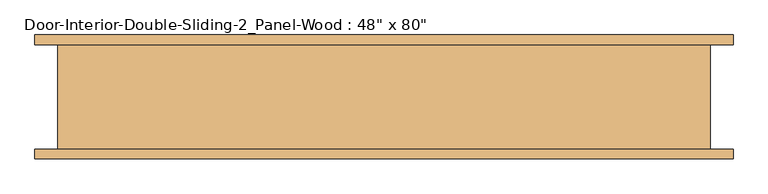
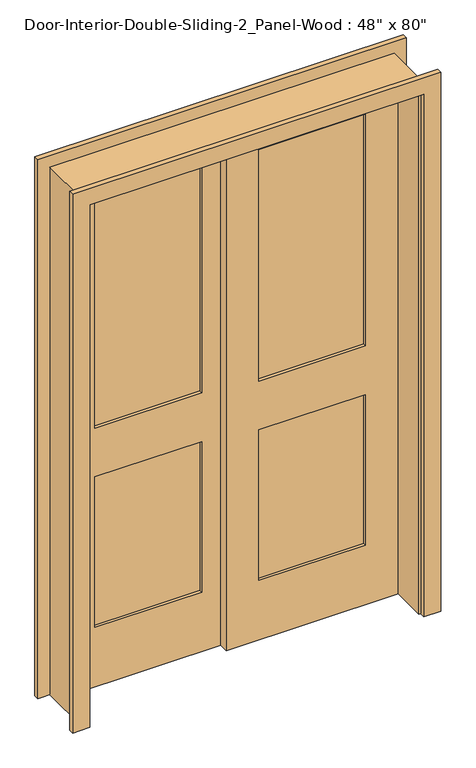
"""IFC4 building model written with IfcOpenShell, lengths in millimetres: door geometry."""

from ifc_helpers import new_model, si_unit, frame, origin, place, context, project, spatial, polyline, outline, extrude, source, transform, mapped, element, save


def door_f9cb40a9(model_context):
    return source(origin(), model_context, "Body", "SweptSolid", [
        extrude(outline(polyline([(488.95, 40.2166667), (95.25, 40.2166667), (95.25, 51.8583333), (488.95, 51.8583333), (488.95, 40.2166667)])), frame((0.0, 0.0, 1009.65), z_axis=(0.0, 0.0, 1.0), x_axis=(1.0, 0.0, 0.0)), (0.0, 0.0, 1.0), 903.2875),
        extrude(outline(polyline([(488.95, 40.2166667), (95.25, 40.2166667), (95.25, 51.8583333), (488.95, 51.8583333), (488.95, 40.2166667)])), frame((0.0, 0.0, 231.775), z_axis=(0.0, 0.0, 1.0), x_axis=(1.0, 0.0, 0.0)), (0.0, 0.0, 1.0), 587.375),
        extrude(outline(polyline([(2032.0, -25.4), (0.0, -25.4), (0.0, 609.6), (2032.0, 609.6), (2032.0, -25.4)]), holes=[polyline([(1912.9375, 95.25), (1912.9375, 488.95), (1009.65, 488.95), (1009.65, 95.25), (1912.9375, 95.25)]), polyline([(819.15, 95.25), (819.15, 488.95), (231.775, 488.95), (231.775, 95.25), (819.15, 95.25)])]), frame((0.0, 28.575, 0.0), z_axis=(0.0, 1.0, 0.0), x_axis=(0.0, 0.0, 1.0)), (0.0, 0.0, 1.0), 34.925),
        extrude(outline(polyline([(-95.25, 75.1416667), (-488.95, 75.1416667), (-488.95, 86.7833333), (-95.25, 86.7833333), (-95.25, 75.1416667)])), frame((0.0, 0.0, 1009.65), z_axis=(0.0, 0.0, 1.0), x_axis=(1.0, 0.0, 0.0)), (0.0, 0.0, 1.0), 903.2875),
        extrude(outline(polyline([(-95.25, 75.1416667), (-488.95, 75.1416667), (-488.95, 86.7833333), (-95.25, 86.7833333), (-95.25, 75.1416667)])), frame((0.0, 0.0, 231.775), z_axis=(0.0, 0.0, 1.0), x_axis=(1.0, 0.0, 0.0)), (0.0, 0.0, 1.0), 587.375),
        extrude(outline(polyline([(2032.0, -609.6), (0.0, -609.6), (0.0, 25.4), (2032.0, 25.4), (2032.0, -609.6)]), holes=[polyline([(1912.9375, -488.95), (1912.9375, -95.25), (1009.65, -95.25), (1009.65, -488.95), (1912.9375, -488.95)]), polyline([(819.15, -488.95), (819.15, -95.25), (231.775, -95.25), (231.775, -488.95), (819.15, -488.95)])]), frame((0.0, 63.5, 0.0), z_axis=(0.0, 1.0, 0.0), x_axis=(0.0, 0.0, 1.0)), (0.0, 0.0, 1.0), 34.925),
        extrude(outline(polyline([(0.0, 609.6), (0.0, 635.0), (2057.4, 635.0), (2057.4, -635.0), (0.0, -635.0), (0.0, -609.6), (2032.0, -609.6), (2032.0, 609.6), (0.0, 609.6)])), frame((0.0, -104.775, 0.0), z_axis=(0.0, 1.0, 0.0), x_axis=(0.0, 0.0, 1.0)), (0.0, 0.0, 1.0), 203.2),
        extrude(outline(polyline([(0.0, 615.95), (0.0, 679.45), (2101.85, 679.45), (2101.85, -679.45), (0.0, -679.45), (0.0, -615.95), (2038.35, -615.95), (2038.35, 615.95), (0.0, 615.95)])), frame((0.0, -123.825, 0.0), z_axis=(0.0, 1.0, 0.0), x_axis=(0.0, 0.0, 1.0)), (0.0, 0.0, 1.0), 19.05),
        extrude(outline(polyline([(0.0, 615.95), (0.0, 679.45), (2101.85, 679.45), (2101.85, -679.45), (0.0, -679.45), (0.0, -615.95), (2038.35, -615.95), (2038.35, 615.95), (0.0, 615.95)])), frame((0.0, 98.425, 0.0), z_axis=(0.0, 1.0, 0.0), x_axis=(0.0, 0.0, 1.0)), (0.0, 0.0, 1.0), 19.05),
    ])


if __name__ == "__main__":
    model = new_model("IFC4")
    model_context = context("Model", 3, world=origin())
    ifc_project = project(units=[si_unit("LENGTHUNIT", "METRE", prefix="MILLI")], contexts=[model_context])
    site = spatial("IfcSite", under=ifc_project)
    building = spatial("IfcBuilding", under=site)
    placement = place(None, origin())
    door_shape = door_f9cb40a9(model_context)
    element("IfcDoor", 1, ObjectType="Door-Interior-Double-Sliding-2_Panel-Wood : 48\" x 80\"", at=placement, inside=building, context=model_context, shape_type="MappedRepresentation", body=[
        mapped(door_shape, transform((0.0, 0.0, 0.0), x_axis=(1.0, 0.0, 0.0), y_axis=(0.0, 1.0, 0.0), z_axis=(0.0, 0.0, 1.0))),
    ])
    save(model, "model.ifc")

# Revit data of these elements
# Type "Door-Interior-Double-Sliding-2_Panel-Wood : 48\" x 80\""
#   Type Mark = "9"
#   Assembly Code = "C1020300"
#   Analytic Construction = "Wooden"
#   Top Rail = 0' - 4 11/16"
#   Thickness = 0' - 1 3/8"
#   Thermal Resistance (R) = 2.5876 (h·ft²·°F)/BTU
#   Stiles = 0' - 4 3/4"
#   Rough Width = 4' - 2"
#   Rough Height = 6' - 9"
#   Lock Rail = 0' - 7 1/2"
#   Height = 6' - 8"
#   Width = 4' - 0"
#   Heat Transfer Coefficient (U) = 0.3865 BTU/(h·ft²·°F)
#   Bottom Rail = 0' - 9 1/8"
#   Trim Material = Cherry
#   Panel Material = Cherry
#   Frame Material = Cherry
#   Visual Light Transmittance = 0
#   Solar Heat Gain Coefficient = 0
#   Wall Closure = (empty or 0)
#   Function = (empty or 0)
# Element 1 (IfcDoor, "Door-Interior-Double-Sliding-2_Panel-Wood : 48\" x 80\"")
#   Materials on its faces: "Cherry"
# Materials
#   "Cherry": class "Wood", colour RGB 226 177 128, transparency 0, Description = "Prunus Serotina", Cost = 0
